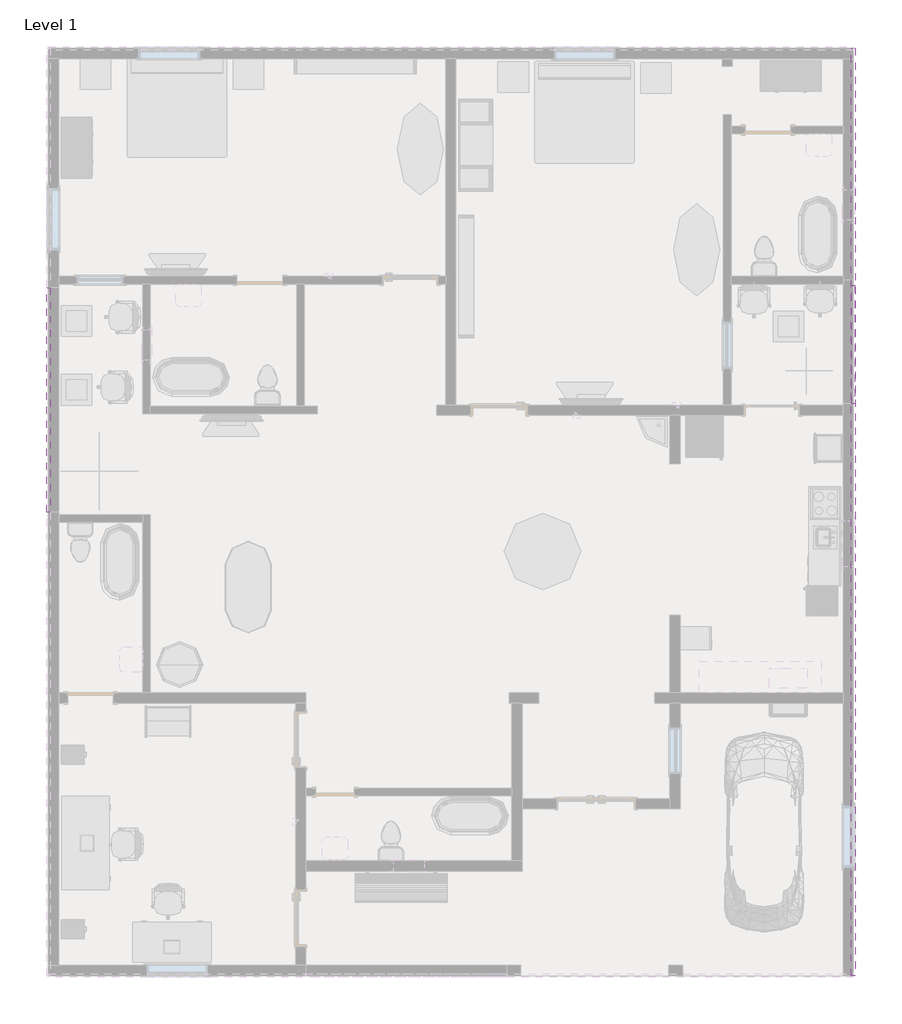
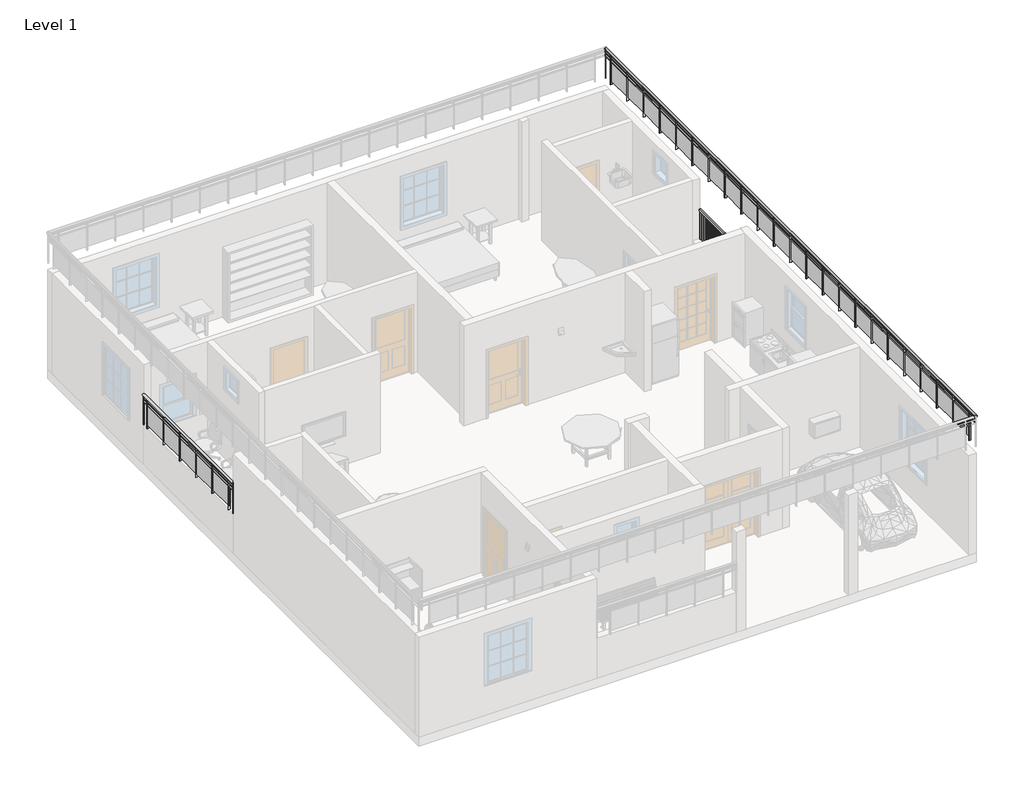
# One storey, part 3 of 4: 3 railings.
"""IFC4 building model written with IfcOpenShell, lengths in millimetres."""

from ifc_helpers import new_model, si_unit, point, frame, origin, place, context, project, spatial, polyline, ellipse_curve, trimmed, outline, extrude, element, save
from ifc_brep_helpers import plane_surface, extruded_surface, advanced_brep

model = new_model("IFC4")

# Units and contexts
model_context = context("Model", 3, world=origin())
ifc_project = project(units=[si_unit("LENGTHUNIT", "METRE", prefix="MILLI")], contexts=[model_context])

# Site, building, storey
site = spatial("IfcSite", under=ifc_project)
building = spatial("IfcBuilding", under=site)
storey = spatial("IfcBuildingStorey", under=building, Name="Level 1", Elevation=0.0)

# Railings
placement = place(None, origin())
element("IfcRailing", 1, ObjectType="Glass Panel - Bottom Fill", at=placement, inside=storey, context=model_context, shape_type="SolidModel", body=[
    advanced_brep(
    [(-17679.8484731, 3327.0442281, 2133.6), (-17603.6484731, 3327.0442281, 2133.6), (-17679.8484731, 7797.4442281, 2133.6), (-17603.6484731, 7797.4442281, 2133.6)],
    [
        (0, 1, ellipse_curve(frame((-17641.7484731, 3327.0442281, 2133.6), z_axis=(0.0, -1.0, 0.0), x_axis=(1.0, 0.0, 0.0)), 38.1, 28.575)),
        (1, 0, ellipse_curve(frame((-17641.7484731, 3327.0442281, 2133.6), z_axis=(0.0, -1.0, 0.0), x_axis=(1.0, 0.0, 0.0)), 38.1, 28.575)),
        (2, 3, ellipse_curve(frame((-17641.7484731, 7797.4442281, 2133.6), z_axis=(0.0, 1.0, 0.0), x_axis=(1.0, 0.0, 0.0)), 38.1, 28.575)),
        (3, 2, ellipse_curve(frame((-17641.7484731, 7797.4442281, 2133.6), z_axis=(0.0, 1.0, 0.0), x_axis=(1.0, 0.0, 0.0)), 38.1, 28.575)),
        (0, 2),
        (3, 1),
    ],
    [
        plane_surface(frame((-17641.7484731, 3327.0442281, 2133.6), z_axis=(0.0, -1.0, 0.0), x_axis=(0.0, 0.0, 1.0))),
        plane_surface(frame((-17641.7484731, 7797.4442281, 2133.6), z_axis=(0.0, 1.0, 0.0), x_axis=(0.0, 0.0, 1.0))),
        extruded_surface(trimmed(ellipse_curve(frame((-17641.7484731, 7797.4442281, 2133.6), z_axis=(0.0, -1.0, 0.0), x_axis=(1.0, 0.0, 0.0)), 38.1, 28.575), [point((-17679.8484731, 7797.4442281, 2133.6))], [point((-17603.6484731, 7797.4442281, 2133.6))], True, "CARTESIAN"), (0.0, -4470.4, 0.0), 4470.4),
        extruded_surface(trimmed(ellipse_curve(frame((-17641.7484731, 7797.4442281, 2133.6), z_axis=(0.0, -1.0, 0.0), x_axis=(1.0, 0.0, 0.0)), 38.1, 28.575), [point((-17603.6484731, 7797.4442281, 2133.6))], [point((-17679.8484731, 7797.4442281, 2133.6))], True, "CARTESIAN"), (0.0, -4470.4, 0.0), 4470.4),
    ],
    [
        (0, [[1, 2]]),
        (1, [[3, 4]]),
        (2, [[-1, 5, -4, 6]]),
        (3, [[-2, -6, -3, -5]]),
    ],
),
    extrude(outline(polyline([(-17629.0484731, 3327.0442281), (-17654.4484731, 3327.0442281), (-17654.4484731, 7797.4442281), (-17629.0484731, 7797.4442281), (-17629.0484731, 3327.0442281)])), frame((0.0, 0.0, 2019.3), z_axis=(0.0, 0.0, 1.0), x_axis=(1.0, 0.0, 0.0)), (0.0, 0.0, 1.0), 25.4),
    extrude(outline(polyline([(-17629.0484731, 3327.0442281), (-17654.4484731, 3327.0442281), (-17654.4484731, 7797.4442281), (-17629.0484731, 7797.4442281), (-17629.0484731, 3327.0442281)])), frame((0.0, 0.0, 1917.7), z_axis=(0.0, 0.0, 1.0), x_axis=(1.0, 0.0, 0.0)), (0.0, 0.0, 1.0), 25.4),
    extrude(outline(polyline([(-17616.3484731, 7587.8942281), (-17667.1484731, 7587.8942281), (-17667.1484731, 7600.5942281), (-17616.3484731, 7600.5942281), (-17616.3484731, 7587.8942281)])), frame((0.0, 0.0, 1219.2), z_axis=(0.0, 0.0, 1.0), x_axis=(1.0, 0.0, 0.0)), (0.0, 0.0, 1.0), 885.6788223),
    extrude(outline(polyline([(-17648.2836301, 6781.4442281), (-17648.2836301, 7594.2442281), (-17641.9336301, 7594.2442281), (-17641.9336301, 6781.4442281), (-17648.2836301, 6781.4442281)])), frame((0.0, 0.0, 1320.8), z_axis=(0.0, 0.0, 1.0), x_axis=(1.0, 0.0, 0.0)), (0.0, 0.0, 1.0), 596.9),
    extrude(outline(polyline([(-17616.3484731, 6775.0942281), (-17667.1484731, 6775.0942281), (-17667.1484731, 6787.7942281), (-17616.3484731, 6787.7942281), (-17616.3484731, 6775.0942281)])), frame((0.0, 0.0, 1219.2), z_axis=(0.0, 0.0, 1.0), x_axis=(1.0, 0.0, 0.0)), (0.0, 0.0, 1.0), 885.6788223),
    extrude(outline(polyline([(-17648.2836301, 5968.6442281), (-17648.2836301, 6781.4442281), (-17641.9336301, 6781.4442281), (-17641.9336301, 5968.6442281), (-17648.2836301, 5968.6442281)])), frame((0.0, 0.0, 1320.8), z_axis=(0.0, 0.0, 1.0), x_axis=(1.0, 0.0, 0.0)), (0.0, 0.0, 1.0), 596.9),
    extrude(outline(polyline([(-17616.3484731, 5962.2942281), (-17667.1484731, 5962.2942281), (-17667.1484731, 5974.9942281), (-17616.3484731, 5974.9942281), (-17616.3484731, 5962.2942281)])), frame((0.0, 0.0, 1219.2), z_axis=(0.0, 0.0, 1.0), x_axis=(1.0, 0.0, 0.0)), (0.0, 0.0, 1.0), 885.6788223),
    extrude(outline(polyline([(-17648.2836301, 5155.8442281), (-17648.2836301, 5968.6442281), (-17641.9336301, 5968.6442281), (-17641.9336301, 5155.8442281), (-17648.2836301, 5155.8442281)])), frame((0.0, 0.0, 1320.8), z_axis=(0.0, 0.0, 1.0), x_axis=(1.0, 0.0, 0.0)), (0.0, 0.0, 1.0), 596.9),
    extrude(outline(polyline([(-17616.3484731, 5149.4942281), (-17667.1484731, 5149.4942281), (-17667.1484731, 5162.1942281), (-17616.3484731, 5162.1942281), (-17616.3484731, 5149.4942281)])), frame((0.0, 0.0, 1219.2), z_axis=(0.0, 0.0, 1.0), x_axis=(1.0, 0.0, 0.0)), (0.0, 0.0, 1.0), 885.6788223),
    extrude(outline(polyline([(-17648.2836301, 4343.0442281), (-17648.2836301, 5155.8442281), (-17641.9336301, 5155.8442281), (-17641.9336301, 4343.0442281), (-17648.2836301, 4343.0442281)])), frame((0.0, 0.0, 1320.8), z_axis=(0.0, 0.0, 1.0), x_axis=(1.0, 0.0, 0.0)), (0.0, 0.0, 1.0), 596.9),
    extrude(outline(polyline([(-17616.3484731, 4336.6942281), (-17667.1484731, 4336.6942281), (-17667.1484731, 4349.3942281), (-17616.3484731, 4349.3942281), (-17616.3484731, 4336.6942281)])), frame((0.0, 0.0, 1219.2), z_axis=(0.0, 0.0, 1.0), x_axis=(1.0, 0.0, 0.0)), (0.0, 0.0, 1.0), 885.6788223),
    extrude(outline(polyline([(-17648.2836301, 3530.2442281), (-17648.2836301, 4343.0442281), (-17641.9336301, 4343.0442281), (-17641.9336301, 3530.2442281), (-17648.2836301, 3530.2442281)])), frame((0.0, 0.0, 1320.8), z_axis=(0.0, 0.0, 1.0), x_axis=(1.0, 0.0, 0.0)), (0.0, 0.0, 1.0), 596.9),
    extrude(outline(polyline([(-17616.3484731, 3523.8942281), (-17667.1484731, 3523.8942281), (-17667.1484731, 3536.5942281), (-17616.3484731, 3536.5942281), (-17616.3484731, 3523.8942281)])), frame((0.0, 0.0, 1219.2), z_axis=(0.0, 0.0, 1.0), x_axis=(1.0, 0.0, 0.0)), (0.0, 0.0, 1.0), 885.6788223),
    extrude(outline(polyline([(-17632.2234731, 7784.7442281), (-17651.2734731, 7784.7442281), (-17651.2734731, 7803.7942281), (-17632.2234731, 7803.7942281), (-17632.2234731, 7784.7442281)])), frame((0.0, 0.0, 1219.2), z_axis=(0.0, 0.0, 1.0), x_axis=(1.0, 0.0, 0.0)), (0.0, 0.0, 1.0), 885.6788223),
    extrude(outline(polyline([(-17632.2234731, 3320.6942281), (-17651.2734731, 3320.6942281), (-17651.2734731, 3339.7442281), (-17632.2234731, 3339.7442281), (-17632.2234731, 3320.6942281)])), frame((0.0, 0.0, 1219.2), z_axis=(0.0, 0.0, 1.0), x_axis=(1.0, 0.0, 0.0)), (0.0, 0.0, 1.0), 885.6788223),
])
element("IfcRailing", 2, ObjectType="Glass Panel - Bottom Fill", at=placement, inside=storey, context=model_context, shape_type="SolidModel", body=[
    advanced_brep(
    [(-1550.8484731, 12572.6442281, 4165.6), (-1627.0484731, 12572.6442281, 4165.6), (-1550.8484731, -5918.5557719, 4165.6), (-1627.0484731, -5918.5557719, 4165.6)],
    [
        (0, 1, ellipse_curve(frame((-1588.9484731, 12572.6442281, 4165.6), z_axis=(0.0, 1.0, 0.0), x_axis=(-1.0, 0.0, 0.0)), 38.1, 28.575)),
        (1, 0, ellipse_curve(frame((-1588.9484731, 12572.6442281, 4165.6), z_axis=(0.0, 1.0, 0.0), x_axis=(-1.0, 0.0, 0.0)), 38.1, 28.575)),
        (2, 3, ellipse_curve(frame((-1588.9484731, -5918.5557719, 4165.6), z_axis=(0.0, -1.0, 0.0), x_axis=(-1.0, 0.0, 0.0)), 38.1, 28.575)),
        (3, 2, ellipse_curve(frame((-1588.9484731, -5918.5557719, 4165.6), z_axis=(0.0, -1.0, 0.0), x_axis=(-1.0, 0.0, 0.0)), 38.1, 28.575)),
        (0, 2),
        (3, 1),
    ],
    [
        plane_surface(frame((-1588.9484731, 12572.6442281, 4165.6), z_axis=(0.0, 1.0, 0.0), x_axis=(0.0, 0.0, -1.0))),
        plane_surface(frame((-1588.9484731, -5918.5557719, 4165.6), z_axis=(0.0, -1.0, 0.0), x_axis=(0.0, 0.0, -1.0))),
        extruded_surface(trimmed(ellipse_curve(frame((-1588.9484731, -5918.5557719, 4165.6), z_axis=(0.0, 1.0, 0.0), x_axis=(-1.0, 0.0, 0.0)), 38.1, 28.575), [point((-1550.8484731, -5918.5557719, 4165.6))], [point((-1627.0484731, -5918.5557719, 4165.6))], True, "CARTESIAN"), (0.0, 18491.2, 0.0), 18491.2),
        extruded_surface(trimmed(ellipse_curve(frame((-1588.9484731, -5918.5557719, 4165.6), z_axis=(0.0, 1.0, 0.0), x_axis=(-1.0, 0.0, 0.0)), 38.1, 28.575), [point((-1627.0484731, -5918.5557719, 4165.6))], [point((-1550.8484731, -5918.5557719, 4165.6))], True, "CARTESIAN"), (0.0, 18491.2, 0.0), 18491.2),
    ],
    [
        (0, [[1, 2]]),
        (1, [[3, 4]]),
        (2, [[-1, 5, -4, 6]]),
        (3, [[-2, -6, -3, -5]]),
    ],
),
    extrude(outline(polyline([(-1601.6484731, 12572.6442281), (-1576.2484731, 12572.6442281), (-1576.2484731, -5918.5557719), (-1601.6484731, -5918.5557719), (-1601.6484731, 12572.6442281)])), frame((0.0, 0.0, 4051.3), z_axis=(0.0, 0.0, 1.0), x_axis=(1.0, 0.0, 0.0)), (0.0, 0.0, 1.0), 25.4),
    extrude(outline(polyline([(-1601.6484731, 12572.6442281), (-1576.2484731, 12572.6442281), (-1576.2484731, -5918.5557719), (-1601.6484731, -5918.5557719), (-1601.6484731, 12572.6442281)])), frame((0.0, 0.0, 3949.7), z_axis=(0.0, 0.0, 1.0), x_axis=(1.0, 0.0, 0.0)), (0.0, 0.0, 1.0), 25.4),
    extrude(outline(polyline([(-1614.3484731, -5607.4057719), (-1563.5484731, -5607.4057719), (-1563.5484731, -5620.1057719), (-1614.3484731, -5620.1057719), (-1614.3484731, -5607.4057719)])), frame((0.0, 0.0, 3251.2), z_axis=(0.0, 0.0, 1.0), x_axis=(1.0, 0.0, 0.0)), (0.0, 0.0, 1.0), 885.6788223),
    extrude(outline(polyline([(-1582.4133161, -4800.9557719), (-1582.4133161, -5613.7557719), (-1588.7633161, -5613.7557719), (-1588.7633161, -4800.9557719), (-1582.4133161, -4800.9557719)])), frame((0.0, 0.0, 3352.8), z_axis=(0.0, 0.0, 1.0), x_axis=(1.0, 0.0, 0.0)), (0.0, 0.0, 1.0), 596.9),
    extrude(outline(polyline([(-1614.3484731, -4794.6057719), (-1563.5484731, -4794.6057719), (-1563.5484731, -4807.3057719), (-1614.3484731, -4807.3057719), (-1614.3484731, -4794.6057719)])), frame((0.0, 0.0, 3251.2), z_axis=(0.0, 0.0, 1.0), x_axis=(1.0, 0.0, 0.0)), (0.0, 0.0, 1.0), 885.6788223),
    extrude(outline(polyline([(-1582.4133161, -3988.1557719), (-1582.4133161, -4800.9557719), (-1588.7633161, -4800.9557719), (-1588.7633161, -3988.1557719), (-1582.4133161, -3988.1557719)])), frame((0.0, 0.0, 3352.8), z_axis=(0.0, 0.0, 1.0), x_axis=(1.0, 0.0, 0.0)), (0.0, 0.0, 1.0), 596.9),
    extrude(outline(polyline([(-1614.3484731, -3981.8057719), (-1563.5484731, -3981.8057719), (-1563.5484731, -3994.5057719), (-1614.3484731, -3994.5057719), (-1614.3484731, -3981.8057719)])), frame((0.0, 0.0, 3251.2), z_axis=(0.0, 0.0, 1.0), x_axis=(1.0, 0.0, 0.0)), (0.0, 0.0, 1.0), 885.6788223),
    extrude(outline(polyline([(-1582.4133161, -3175.3557719), (-1582.4133161, -3988.1557719), (-1588.7633161, -3988.1557719), (-1588.7633161, -3175.3557719), (-1582.4133161, -3175.3557719)])), frame((0.0, 0.0, 3352.8), z_axis=(0.0, 0.0, 1.0), x_axis=(1.0, 0.0, 0.0)), (0.0, 0.0, 1.0), 596.9),
    extrude(outline(polyline([(-1614.3484731, -3169.0057719), (-1563.5484731, -3169.0057719), (-1563.5484731, -3181.7057719), (-1614.3484731, -3181.7057719), (-1614.3484731, -3169.0057719)])), frame((0.0, 0.0, 3251.2), z_axis=(0.0, 0.0, 1.0), x_axis=(1.0, 0.0, 0.0)), (0.0, 0.0, 1.0), 885.6788223),
    extrude(outline(polyline([(-1582.4133161, -2362.5557719), (-1582.4133161, -3175.3557719), (-1588.7633161, -3175.3557719), (-1588.7633161, -2362.5557719), (-1582.4133161, -2362.5557719)])), frame((0.0, 0.0, 3352.8), z_axis=(0.0, 0.0, 1.0), x_axis=(1.0, 0.0, 0.0)), (0.0, 0.0, 1.0), 596.9),
    extrude(outline(polyline([(-1614.3484731, -2356.2057719), (-1563.5484731, -2356.2057719), (-1563.5484731, -2368.9057719), (-1614.3484731, -2368.9057719), (-1614.3484731, -2356.2057719)])), frame((0.0, 0.0, 3251.2), z_axis=(0.0, 0.0, 1.0), x_axis=(1.0, 0.0, 0.0)), (0.0, 0.0, 1.0), 885.6788223),
    extrude(outline(polyline([(-1582.4133161, -1549.7557719), (-1582.4133161, -2362.5557719), (-1588.7633161, -2362.5557719), (-1588.7633161, -1549.7557719), (-1582.4133161, -1549.7557719)])), frame((0.0, 0.0, 3352.8), z_axis=(0.0, 0.0, 1.0), x_axis=(1.0, 0.0, 0.0)), (0.0, 0.0, 1.0), 596.9),
    extrude(outline(polyline([(-1614.3484731, -1543.4057719), (-1563.5484731, -1543.4057719), (-1563.5484731, -1556.1057719), (-1614.3484731, -1556.1057719), (-1614.3484731, -1543.4057719)])), frame((0.0, 0.0, 3251.2), z_axis=(0.0, 0.0, 1.0), x_axis=(1.0, 0.0, 0.0)), (0.0, 0.0, 1.0), 885.6788223),
    extrude(outline(polyline([(-1582.4133161, -736.9557719), (-1582.4133161, -1549.7557719), (-1588.7633161, -1549.7557719), (-1588.7633161, -736.9557719), (-1582.4133161, -736.9557719)])), frame((0.0, 0.0, 3352.8), z_axis=(0.0, 0.0, 1.0), x_axis=(1.0, 0.0, 0.0)), (0.0, 0.0, 1.0), 596.9),
    extrude(outline(polyline([(-1614.3484731, -730.6057719), (-1563.5484731, -730.6057719), (-1563.5484731, -743.3057719), (-1614.3484731, -743.3057719), (-1614.3484731, -730.6057719)])), frame((0.0, 0.0, 3251.2), z_axis=(0.0, 0.0, 1.0), x_axis=(1.0, 0.0, 0.0)), (0.0, 0.0, 1.0), 885.6788223),
    extrude(outline(polyline([(-1582.4133161, 75.8442281), (-1582.4133161, -736.9557719), (-1588.7633161, -736.9557719), (-1588.7633161, 75.8442281), (-1582.4133161, 75.8442281)])), frame((0.0, 0.0, 3352.8), z_axis=(0.0, 0.0, 1.0), x_axis=(1.0, 0.0, 0.0)), (0.0, 0.0, 1.0), 596.9),
    extrude(outline(polyline([(-1614.3484731, 82.1942281), (-1563.5484731, 82.1942281), (-1563.5484731, 69.4942281), (-1614.3484731, 69.4942281), (-1614.3484731, 82.1942281)])), frame((0.0, 0.0, 3251.2), z_axis=(0.0, 0.0, 1.0), x_axis=(1.0, 0.0, 0.0)), (0.0, 0.0, 1.0), 885.6788223),
    extrude(outline(polyline([(-1582.4133161, 888.6442281), (-1582.4133161, 75.8442281), (-1588.7633161, 75.8442281), (-1588.7633161, 888.6442281), (-1582.4133161, 888.6442281)])), frame((0.0, 0.0, 3352.8), z_axis=(0.0, 0.0, 1.0), x_axis=(1.0, 0.0, 0.0)), (0.0, 0.0, 1.0), 596.9),
    extrude(outline(polyline([(-1614.3484731, 894.9942281), (-1563.5484731, 894.9942281), (-1563.5484731, 882.2942281), (-1614.3484731, 882.2942281), (-1614.3484731, 894.9942281)])), frame((0.0, 0.0, 3251.2), z_axis=(0.0, 0.0, 1.0), x_axis=(1.0, 0.0, 0.0)), (0.0, 0.0, 1.0), 885.6788223),
    extrude(outline(polyline([(-1582.4133161, 1701.4442281), (-1582.4133161, 888.6442281), (-1588.7633161, 888.6442281), (-1588.7633161, 1701.4442281), (-1582.4133161, 1701.4442281)])), frame((0.0, 0.0, 3352.8), z_axis=(0.0, 0.0, 1.0), x_axis=(1.0, 0.0, 0.0)), (0.0, 0.0, 1.0), 596.9),
    extrude(outline(polyline([(-1614.3484731, 1707.7942281), (-1563.5484731, 1707.7942281), (-1563.5484731, 1695.0942281), (-1614.3484731, 1695.0942281), (-1614.3484731, 1707.7942281)])), frame((0.0, 0.0, 3251.2), z_axis=(0.0, 0.0, 1.0), x_axis=(1.0, 0.0, 0.0)), (0.0, 0.0, 1.0), 885.6788223),
    extrude(outline(polyline([(-1582.4133161, 2514.2442281), (-1582.4133161, 1701.4442281), (-1588.7633161, 1701.4442281), (-1588.7633161, 2514.2442281), (-1582.4133161, 2514.2442281)])), frame((0.0, 0.0, 3352.8), z_axis=(0.0, 0.0, 1.0), x_axis=(1.0, 0.0, 0.0)), (0.0, 0.0, 1.0), 596.9),
    extrude(outline(polyline([(-1614.3484731, 2520.5942281), (-1563.5484731, 2520.5942281), (-1563.5484731, 2507.8942281), (-1614.3484731, 2507.8942281), (-1614.3484731, 2520.5942281)])), frame((0.0, 0.0, 3251.2), z_axis=(0.0, 0.0, 1.0), x_axis=(1.0, 0.0, 0.0)), (0.0, 0.0, 1.0), 885.6788223),
    extrude(outline(polyline([(-1582.4133161, 3327.0442281), (-1582.4133161, 2514.2442281), (-1588.7633161, 2514.2442281), (-1588.7633161, 3327.0442281), (-1582.4133161, 3327.0442281)])), frame((0.0, 0.0, 3352.8), z_axis=(0.0, 0.0, 1.0), x_axis=(1.0, 0.0, 0.0)), (0.0, 0.0, 1.0), 596.9),
    extrude(outline(polyline([(-1614.3484731, 3333.3942281), (-1563.5484731, 3333.3942281), (-1563.5484731, 3320.6942281), (-1614.3484731, 3320.6942281), (-1614.3484731, 3333.3942281)])), frame((0.0, 0.0, 3251.2), z_axis=(0.0, 0.0, 1.0), x_axis=(1.0, 0.0, 0.0)), (0.0, 0.0, 1.0), 885.6788223),
    extrude(outline(polyline([(-1582.4133161, 4139.8442281), (-1582.4133161, 3327.0442281), (-1588.7633161, 3327.0442281), (-1588.7633161, 4139.8442281), (-1582.4133161, 4139.8442281)])), frame((0.0, 0.0, 3352.8), z_axis=(0.0, 0.0, 1.0), x_axis=(1.0, 0.0, 0.0)), (0.0, 0.0, 1.0), 596.9),
    extrude(outline(polyline([(-1614.3484731, 4146.1942281), (-1563.5484731, 4146.1942281), (-1563.5484731, 4133.4942281), (-1614.3484731, 4133.4942281), (-1614.3484731, 4146.1942281)])), frame((0.0, 0.0, 3251.2), z_axis=(0.0, 0.0, 1.0), x_axis=(1.0, 0.0, 0.0)), (0.0, 0.0, 1.0), 885.6788223),
    extrude(outline(polyline([(-1582.4133161, 4952.6442281), (-1582.4133161, 4139.8442281), (-1588.7633161, 4139.8442281), (-1588.7633161, 4952.6442281), (-1582.4133161, 4952.6442281)])), frame((0.0, 0.0, 3352.8), z_axis=(0.0, 0.0, 1.0), x_axis=(1.0, 0.0, 0.0)), (0.0, 0.0, 1.0), 596.9),
    extrude(outline(polyline([(-1614.3484731, 4958.9942281), (-1563.5484731, 4958.9942281), (-1563.5484731, 4946.2942281), (-1614.3484731, 4946.2942281), (-1614.3484731, 4958.9942281)])), frame((0.0, 0.0, 3251.2), z_axis=(0.0, 0.0, 1.0), x_axis=(1.0, 0.0, 0.0)), (0.0, 0.0, 1.0), 885.6788223),
    extrude(outline(polyline([(-1582.4133161, 5765.4442281), (-1582.4133161, 4952.6442281), (-1588.7633161, 4952.6442281), (-1588.7633161, 5765.4442281), (-1582.4133161, 5765.4442281)])), frame((0.0, 0.0, 3352.8), z_axis=(0.0, 0.0, 1.0), x_axis=(1.0, 0.0, 0.0)), (0.0, 0.0, 1.0), 596.9),
    extrude(outline(polyline([(-1614.3484731, 5771.7942281), (-1563.5484731, 5771.7942281), (-1563.5484731, 5759.0942281), (-1614.3484731, 5759.0942281), (-1614.3484731, 5771.7942281)])), frame((0.0, 0.0, 3251.2), z_axis=(0.0, 0.0, 1.0), x_axis=(1.0, 0.0, 0.0)), (0.0, 0.0, 1.0), 885.6788223),
    extrude(outline(polyline([(-1582.4133161, 6578.2442281), (-1582.4133161, 5765.4442281), (-1588.7633161, 5765.4442281), (-1588.7633161, 6578.2442281), (-1582.4133161, 6578.2442281)])), frame((0.0, 0.0, 3352.8), z_axis=(0.0, 0.0, 1.0), x_axis=(1.0, 0.0, 0.0)), (0.0, 0.0, 1.0), 596.9),
    extrude(outline(polyline([(-1614.3484731, 6584.5942281), (-1563.5484731, 6584.5942281), (-1563.5484731, 6571.8942281), (-1614.3484731, 6571.8942281), (-1614.3484731, 6584.5942281)])), frame((0.0, 0.0, 3251.2), z_axis=(0.0, 0.0, 1.0), x_axis=(1.0, 0.0, 0.0)), (0.0, 0.0, 1.0), 885.6788223),
    extrude(outline(polyline([(-1582.4133161, 7391.0442281), (-1582.4133161, 6578.2442281), (-1588.7633161, 6578.2442281), (-1588.7633161, 7391.0442281), (-1582.4133161, 7391.0442281)])), frame((0.0, 0.0, 3352.8), z_axis=(0.0, 0.0, 1.0), x_axis=(1.0, 0.0, 0.0)), (0.0, 0.0, 1.0), 596.9),
    extrude(outline(polyline([(-1614.3484731, 7397.3942281), (-1563.5484731, 7397.3942281), (-1563.5484731, 7384.6942281), (-1614.3484731, 7384.6942281), (-1614.3484731, 7397.3942281)])), frame((0.0, 0.0, 3251.2), z_axis=(0.0, 0.0, 1.0), x_axis=(1.0, 0.0, 0.0)), (0.0, 0.0, 1.0), 885.6788223),
    extrude(outline(polyline([(-1582.4133161, 8203.8442281), (-1582.4133161, 7391.0442281), (-1588.7633161, 7391.0442281), (-1588.7633161, 8203.8442281), (-1582.4133161, 8203.8442281)])), frame((0.0, 0.0, 3352.8), z_axis=(0.0, 0.0, 1.0), x_axis=(1.0, 0.0, 0.0)), (0.0, 0.0, 1.0), 596.9),
    extrude(outline(polyline([(-1614.3484731, 8210.1942281), (-1563.5484731, 8210.1942281), (-1563.5484731, 8197.4942281), (-1614.3484731, 8197.4942281), (-1614.3484731, 8210.1942281)])), frame((0.0, 0.0, 3251.2), z_axis=(0.0, 0.0, 1.0), x_axis=(1.0, 0.0, 0.0)), (0.0, 0.0, 1.0), 885.6788223),
    extrude(outline(polyline([(-1582.4133161, 9016.6442281), (-1582.4133161, 8203.8442281), (-1588.7633161, 8203.8442281), (-1588.7633161, 9016.6442281), (-1582.4133161, 9016.6442281)])), frame((0.0, 0.0, 3352.8), z_axis=(0.0, 0.0, 1.0), x_axis=(1.0, 0.0, 0.0)), (0.0, 0.0, 1.0), 596.9),
    extrude(outline(polyline([(-1614.3484731, 9022.9942281), (-1563.5484731, 9022.9942281), (-1563.5484731, 9010.2942281), (-1614.3484731, 9010.2942281), (-1614.3484731, 9022.9942281)])), frame((0.0, 0.0, 3251.2), z_axis=(0.0, 0.0, 1.0), x_axis=(1.0, 0.0, 0.0)), (0.0, 0.0, 1.0), 885.6788223),
    extrude(outline(polyline([(-1582.4133161, 9829.4442281), (-1582.4133161, 9016.6442281), (-1588.7633161, 9016.6442281), (-1588.7633161, 9829.4442281), (-1582.4133161, 9829.4442281)])), frame((0.0, 0.0, 3352.8), z_axis=(0.0, 0.0, 1.0), x_axis=(1.0, 0.0, 0.0)), (0.0, 0.0, 1.0), 596.9),
    extrude(outline(polyline([(-1614.3484731, 9835.7942281), (-1563.5484731, 9835.7942281), (-1563.5484731, 9823.0942281), (-1614.3484731, 9823.0942281), (-1614.3484731, 9835.7942281)])), frame((0.0, 0.0, 3251.2), z_axis=(0.0, 0.0, 1.0), x_axis=(1.0, 0.0, 0.0)), (0.0, 0.0, 1.0), 885.6788223),
    extrude(outline(polyline([(-1582.4133161, 10642.2442281), (-1582.4133161, 9829.4442281), (-1588.7633161, 9829.4442281), (-1588.7633161, 10642.2442281), (-1582.4133161, 10642.2442281)])), frame((0.0, 0.0, 3352.8), z_axis=(0.0, 0.0, 1.0), x_axis=(1.0, 0.0, 0.0)), (0.0, 0.0, 1.0), 596.9),
    extrude(outline(polyline([(-1614.3484731, 10648.5942281), (-1563.5484731, 10648.5942281), (-1563.5484731, 10635.8942281), (-1614.3484731, 10635.8942281), (-1614.3484731, 10648.5942281)])), frame((0.0, 0.0, 3251.2), z_axis=(0.0, 0.0, 1.0), x_axis=(1.0, 0.0, 0.0)), (0.0, 0.0, 1.0), 885.6788223),
    extrude(outline(polyline([(-1582.4133161, 11455.0442281), (-1582.4133161, 10642.2442281), (-1588.7633161, 10642.2442281), (-1588.7633161, 11455.0442281), (-1582.4133161, 11455.0442281)])), frame((0.0, 0.0, 3352.8), z_axis=(0.0, 0.0, 1.0), x_axis=(1.0, 0.0, 0.0)), (0.0, 0.0, 1.0), 596.9),
    extrude(outline(polyline([(-1614.3484731, 11461.3942281), (-1563.5484731, 11461.3942281), (-1563.5484731, 11448.6942281), (-1614.3484731, 11448.6942281), (-1614.3484731, 11461.3942281)])), frame((0.0, 0.0, 3251.2), z_axis=(0.0, 0.0, 1.0), x_axis=(1.0, 0.0, 0.0)), (0.0, 0.0, 1.0), 885.6788223),
    extrude(outline(polyline([(-1582.4133161, 12267.8442281), (-1582.4133161, 11455.0442281), (-1588.7633161, 11455.0442281), (-1588.7633161, 12267.8442281), (-1582.4133161, 12267.8442281)])), frame((0.0, 0.0, 3352.8), z_axis=(0.0, 0.0, 1.0), x_axis=(1.0, 0.0, 0.0)), (0.0, 0.0, 1.0), 596.9),
    extrude(outline(polyline([(-1614.3484731, 12274.1942281), (-1563.5484731, 12274.1942281), (-1563.5484731, 12261.4942281), (-1614.3484731, 12261.4942281), (-1614.3484731, 12274.1942281)])), frame((0.0, 0.0, 3251.2), z_axis=(0.0, 0.0, 1.0), x_axis=(1.0, 0.0, 0.0)), (0.0, 0.0, 1.0), 885.6788223),
    extrude(outline(polyline([(-1598.4734731, -5905.8557719), (-1579.4234731, -5905.8557719), (-1579.4234731, -5924.9057719), (-1598.4734731, -5924.9057719), (-1598.4734731, -5905.8557719)])), frame((0.0, 0.0, 3251.2), z_axis=(0.0, 0.0, 1.0), x_axis=(1.0, 0.0, 0.0)), (0.0, 0.0, 1.0), 885.6788223),
    extrude(outline(polyline([(-1598.4734731, 12578.9942281), (-1579.4234731, 12578.9942281), (-1579.4234731, 12559.9442281), (-1598.4734731, 12559.9442281), (-1598.4734731, 12578.9942281)])), frame((0.0, 0.0, 3251.2), z_axis=(0.0, 0.0, 1.0), x_axis=(1.0, 0.0, 0.0)), (0.0, 0.0, 1.0), 885.6788223),
])
element("IfcRailing", 3, ObjectType="Handrail - Rectangular", at=placement, inside=storey, context=model_context, shape_type="SweptSolid", body=[
    extrude(outline(polyline([(-1563.5484731, 5486.0442281), (-1614.3484731, 5486.0442281), (-1614.3484731, 7848.2442281), (-1563.5484731, 7848.2442281), (-1563.5484731, 5486.0442281)])), frame((0.0, 0.0, 2082.8), z_axis=(0.0, 0.0, 1.0), x_axis=(1.0, 0.0, 0.0)), (0.0, 0.0, 1.0), 50.8),
    extrude(outline(polyline([(-1579.4234731, 7813.3192281), (-1598.4734731, 7813.3192281), (-1598.4734731, 7832.3692281), (-1579.4234731, 7832.3692281), (-1579.4234731, 7813.3192281)])), frame((0.0, 0.0, 1219.2), z_axis=(0.0, 0.0, 1.0), x_axis=(1.0, 0.0, 0.0)), (0.0, 0.0, 1.0), 863.6),
    extrude(outline(polyline([(-1579.4234731, 7711.7192281), (-1598.4734731, 7711.7192281), (-1598.4734731, 7730.7692281), (-1579.4234731, 7730.7692281), (-1579.4234731, 7711.7192281)])), frame((0.0, 0.0, 1219.2), z_axis=(0.0, 0.0, 1.0), x_axis=(1.0, 0.0, 0.0)), (0.0, 0.0, 1.0), 863.6),
    extrude(outline(polyline([(-1579.4234731, 7610.1192281), (-1598.4734731, 7610.1192281), (-1598.4734731, 7629.1692281), (-1579.4234731, 7629.1692281), (-1579.4234731, 7610.1192281)])), frame((0.0, 0.0, 1219.2), z_axis=(0.0, 0.0, 1.0), x_axis=(1.0, 0.0, 0.0)), (0.0, 0.0, 1.0), 863.6),
    extrude(outline(polyline([(-1579.4234731, 7508.5192281), (-1598.4734731, 7508.5192281), (-1598.4734731, 7527.5692281), (-1579.4234731, 7527.5692281), (-1579.4234731, 7508.5192281)])), frame((0.0, 0.0, 1219.2), z_axis=(0.0, 0.0, 1.0), x_axis=(1.0, 0.0, 0.0)), (0.0, 0.0, 1.0), 863.6),
    extrude(outline(polyline([(-1579.4234731, 7406.9192281), (-1598.4734731, 7406.9192281), (-1598.4734731, 7425.9692281), (-1579.4234731, 7425.9692281), (-1579.4234731, 7406.9192281)])), frame((0.0, 0.0, 1219.2), z_axis=(0.0, 0.0, 1.0), x_axis=(1.0, 0.0, 0.0)), (0.0, 0.0, 1.0), 863.6),
    extrude(outline(polyline([(-1579.4234731, 7305.3192281), (-1598.4734731, 7305.3192281), (-1598.4734731, 7324.3692281), (-1579.4234731, 7324.3692281), (-1579.4234731, 7305.3192281)])), frame((0.0, 0.0, 1219.2), z_axis=(0.0, 0.0, 1.0), x_axis=(1.0, 0.0, 0.0)), (0.0, 0.0, 1.0), 863.6),
    extrude(outline(polyline([(-1579.4234731, 7203.7192281), (-1598.4734731, 7203.7192281), (-1598.4734731, 7222.7692281), (-1579.4234731, 7222.7692281), (-1579.4234731, 7203.7192281)])), frame((0.0, 0.0, 1219.2), z_axis=(0.0, 0.0, 1.0), x_axis=(1.0, 0.0, 0.0)), (0.0, 0.0, 1.0), 863.6),
    extrude(outline(polyline([(-1579.4234731, 7102.1192281), (-1598.4734731, 7102.1192281), (-1598.4734731, 7121.1692281), (-1579.4234731, 7121.1692281), (-1579.4234731, 7102.1192281)])), frame((0.0, 0.0, 1219.2), z_axis=(0.0, 0.0, 1.0), x_axis=(1.0, 0.0, 0.0)), (0.0, 0.0, 1.0), 863.6),
    extrude(outline(polyline([(-1579.4234731, 7000.5192281), (-1598.4734731, 7000.5192281), (-1598.4734731, 7019.5692281), (-1579.4234731, 7019.5692281), (-1579.4234731, 7000.5192281)])), frame((0.0, 0.0, 1219.2), z_axis=(0.0, 0.0, 1.0), x_axis=(1.0, 0.0, 0.0)), (0.0, 0.0, 1.0), 863.6),
    extrude(outline(polyline([(-1579.4234731, 6898.9192281), (-1598.4734731, 6898.9192281), (-1598.4734731, 6917.9692281), (-1579.4234731, 6917.9692281), (-1579.4234731, 6898.9192281)])), frame((0.0, 0.0, 1219.2), z_axis=(0.0, 0.0, 1.0), x_axis=(1.0, 0.0, 0.0)), (0.0, 0.0, 1.0), 863.6),
    extrude(outline(polyline([(-1579.4234731, 6797.3192281), (-1598.4734731, 6797.3192281), (-1598.4734731, 6816.3692281), (-1579.4234731, 6816.3692281), (-1579.4234731, 6797.3192281)])), frame((0.0, 0.0, 1219.2), z_axis=(0.0, 0.0, 1.0), x_axis=(1.0, 0.0, 0.0)), (0.0, 0.0, 1.0), 863.6),
    extrude(outline(polyline([(-1579.4234731, 6695.7192281), (-1598.4734731, 6695.7192281), (-1598.4734731, 6714.7692281), (-1579.4234731, 6714.7692281), (-1579.4234731, 6695.7192281)])), frame((0.0, 0.0, 1219.2), z_axis=(0.0, 0.0, 1.0), x_axis=(1.0, 0.0, 0.0)), (0.0, 0.0, 1.0), 863.6),
    extrude(outline(polyline([(-1579.4234731, 6594.1192281), (-1598.4734731, 6594.1192281), (-1598.4734731, 6613.1692281), (-1579.4234731, 6613.1692281), (-1579.4234731, 6594.1192281)])), frame((0.0, 0.0, 1219.2), z_axis=(0.0, 0.0, 1.0), x_axis=(1.0, 0.0, 0.0)), (0.0, 0.0, 1.0), 863.6),
    extrude(outline(polyline([(-1579.4234731, 6492.5192281), (-1598.4734731, 6492.5192281), (-1598.4734731, 6511.5692281), (-1579.4234731, 6511.5692281), (-1579.4234731, 6492.5192281)])), frame((0.0, 0.0, 1219.2), z_axis=(0.0, 0.0, 1.0), x_axis=(1.0, 0.0, 0.0)), (0.0, 0.0, 1.0), 863.6),
    extrude(outline(polyline([(-1579.4234731, 6390.9192281), (-1598.4734731, 6390.9192281), (-1598.4734731, 6409.9692281), (-1579.4234731, 6409.9692281), (-1579.4234731, 6390.9192281)])), frame((0.0, 0.0, 1219.2), z_axis=(0.0, 0.0, 1.0), x_axis=(1.0, 0.0, 0.0)), (0.0, 0.0, 1.0), 863.6),
    extrude(outline(polyline([(-1579.4234731, 6289.3192281), (-1598.4734731, 6289.3192281), (-1598.4734731, 6308.3692281), (-1579.4234731, 6308.3692281), (-1579.4234731, 6289.3192281)])), frame((0.0, 0.0, 1219.2), z_axis=(0.0, 0.0, 1.0), x_axis=(1.0, 0.0, 0.0)), (0.0, 0.0, 1.0), 863.6),
    extrude(outline(polyline([(-1579.4234731, 6187.7192281), (-1598.4734731, 6187.7192281), (-1598.4734731, 6206.7692281), (-1579.4234731, 6206.7692281), (-1579.4234731, 6187.7192281)])), frame((0.0, 0.0, 1219.2), z_axis=(0.0, 0.0, 1.0), x_axis=(1.0, 0.0, 0.0)), (0.0, 0.0, 1.0), 863.6),
    extrude(outline(polyline([(-1579.4234731, 6086.1192281), (-1598.4734731, 6086.1192281), (-1598.4734731, 6105.1692281), (-1579.4234731, 6105.1692281), (-1579.4234731, 6086.1192281)])), frame((0.0, 0.0, 1219.2), z_axis=(0.0, 0.0, 1.0), x_axis=(1.0, 0.0, 0.0)), (0.0, 0.0, 1.0), 863.6),
    extrude(outline(polyline([(-1579.4234731, 5984.5192281), (-1598.4734731, 5984.5192281), (-1598.4734731, 6003.5692281), (-1579.4234731, 6003.5692281), (-1579.4234731, 5984.5192281)])), frame((0.0, 0.0, 1219.2), z_axis=(0.0, 0.0, 1.0), x_axis=(1.0, 0.0, 0.0)), (0.0, 0.0, 1.0), 863.6),
    extrude(outline(polyline([(-1579.4234731, 5882.9192281), (-1598.4734731, 5882.9192281), (-1598.4734731, 5901.9692281), (-1579.4234731, 5901.9692281), (-1579.4234731, 5882.9192281)])), frame((0.0, 0.0, 1219.2), z_axis=(0.0, 0.0, 1.0), x_axis=(1.0, 0.0, 0.0)), (0.0, 0.0, 1.0), 863.6),
    extrude(outline(polyline([(-1579.4234731, 5781.3192281), (-1598.4734731, 5781.3192281), (-1598.4734731, 5800.3692281), (-1579.4234731, 5800.3692281), (-1579.4234731, 5781.3192281)])), frame((0.0, 0.0, 1219.2), z_axis=(0.0, 0.0, 1.0), x_axis=(1.0, 0.0, 0.0)), (0.0, 0.0, 1.0), 863.6),
    extrude(outline(polyline([(-1579.4234731, 5679.7192281), (-1598.4734731, 5679.7192281), (-1598.4734731, 5698.7692281), (-1579.4234731, 5698.7692281), (-1579.4234731, 5679.7192281)])), frame((0.0, 0.0, 1219.2), z_axis=(0.0, 0.0, 1.0), x_axis=(1.0, 0.0, 0.0)), (0.0, 0.0, 1.0), 863.6),
    extrude(outline(polyline([(-1579.4234731, 5578.1192281), (-1598.4734731, 5578.1192281), (-1598.4734731, 5597.1692281), (-1579.4234731, 5597.1692281), (-1579.4234731, 5578.1192281)])), frame((0.0, 0.0, 1219.2), z_axis=(0.0, 0.0, 1.0), x_axis=(1.0, 0.0, 0.0)), (0.0, 0.0, 1.0), 863.6),
    extrude(outline(polyline([(-1579.4234731, 7829.1942281), (-1598.4734731, 7829.1942281), (-1598.4734731, 7848.2442281), (-1579.4234731, 7848.2442281), (-1579.4234731, 7829.1942281)])), frame((0.0, 0.0, 1219.2), z_axis=(0.0, 0.0, 1.0), x_axis=(1.0, 0.0, 0.0)), (0.0, 0.0, 1.0), 863.6),
    extrude(outline(polyline([(-1579.4234731, 5486.0442281), (-1598.4734731, 5486.0442281), (-1598.4734731, 5505.0942281), (-1579.4234731, 5505.0942281), (-1579.4234731, 5486.0442281)])), frame((0.0, 0.0, 1219.2), z_axis=(0.0, 0.0, 1.0), x_axis=(1.0, 0.0, 0.0)), (0.0, 0.0, 1.0), 863.6),
])

save(model, "model.ifc")

# Revit data of these elements
# Type "Glass Panel - Bottom Fill"
#   Assembly Code = "C2010400"
#   built-in parameter 1008612 = 0.0416667 (stored number, unit not read)
#   built-in parameter 1008611 = 0.0416667 (stored number, unit not read)
#   built-in parameter 1008609 = 0.333333 (stored number, unit not read)
#   built-in parameter 1008604 = 0.166667 (stored number, unit not read)
#   built-in parameter 1008603 = 0.166667 (stored number, unit not read)
#   Railing Height = 3' - 0"
#   built-in parameter 1008630 = 2
#   built-in parameter 1008610 = 2
#   built-in parameter 1008618 = Baluster - Square : 3/4"
# Type "Handrail - Rectangular"
#   Assembly Code = "C2010400"
#   built-in parameter 1008612 = 0.0416667 (stored number, unit not read)
#   built-in parameter 1008611 = 0.0416667 (stored number, unit not read)
#   built-in parameter 1008609 = 0.333333 (stored number, unit not read)
#   built-in parameter 1008604 = 0.166667 (stored number, unit not read)
#   built-in parameter 1008603 = 0.166667 (stored number, unit not read)
#   Railing Height = 3' - 0"
#   built-in parameter 1008630 = 2
#   built-in parameter 1008610 = 2
#   built-in parameter 1008618 = Baluster - Square : 3/4"
# Element 1 (IfcRailing, "Glass Panel - Bottom Fill")
#   built-in parameter 1008621 = 4 (stored number, unit not read)
#   Phase Created = New Construction
#   Materials on its faces: "Glass"
# Element 2 (IfcRailing, "Glass Panel - Bottom Fill")
#   built-in parameter 1008621 = 10.6667 (stored number, unit not read)
#   Phase Created = New Construction
#   Materials on its faces: "Glass"
# Element 3 (IfcRailing, "Handrail - Rectangular")
#   built-in parameter 1008621 = 4 (stored number, unit not read)
#   Phase Created = New Construction
# Materials
#   "Glass": class "Glass", colour RGB 0 128 192, transparency 0.75, Description = "Soda Lime Glass", Cost = 0
